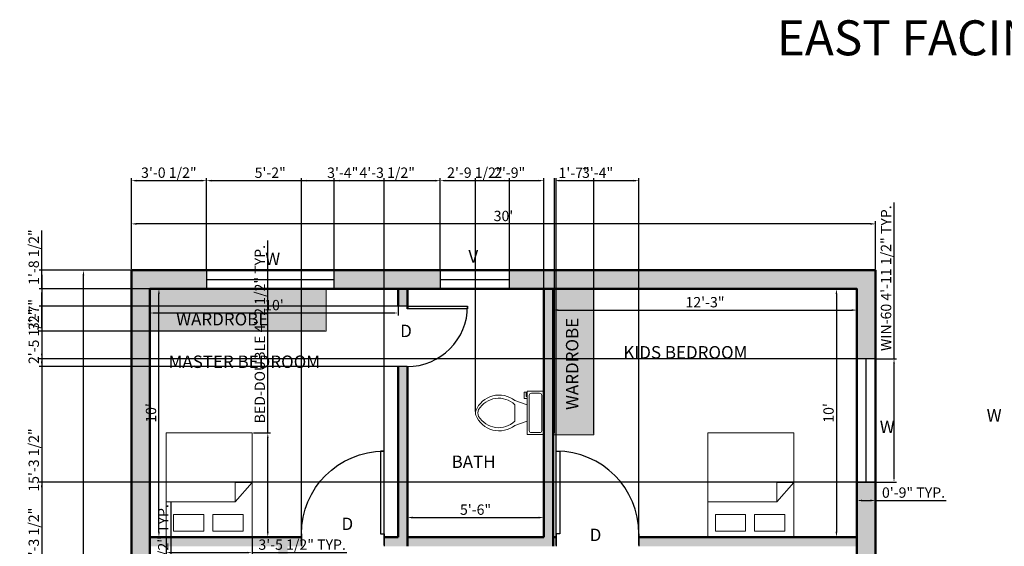
# Model space of a CAD drawing. Units: inches. Extents: x 2064 to 2999, y 1440 to 2089.
# Tile 4 of 7: x 2064 to 2540, y 1835 to 2089. Entities that reach past the tile are written whole.
import ezdxf

# ---------------------------------------------------------------- set-up
doc = ezdxf.new("R2010")
doc.units = ezdxf.units.IN
for name, color, linetype, lineweight in [('A-ANNO-DIMS', 2, 'Continuous', 18), ('A-ANNO-TEXT', 3, 'Continuous', 18), ('A-AREA-IDEN', 7, 'Continuous', 18), ('A-DOOR', 4, 'Continuous', 25), ('A-FLOR-FIXT', 9, 'Continuous', 18), ('A-FURN', 8, 'Continuous', 18), ('A-FURN-PATT', 252, 'Continuous', 13), ('A-GLAZ', 3, 'Continuous', 25), ('A-WALL', 7, 'Continuous', 50), ('A-WALL-PATT', 8, 'Continuous', 13)]:
    doc.layers.add(name, color=color, linetype=linetype, lineweight=lineweight)
doc.styles.get("Standard").update_dxf_attribs({"font": 'arial.ttf'})
doc.dimstyles.new('ISO-25', dxfattribs={"dimtxt": 5, "dimasz": 2.5, "dimexe": 1.25, "dimexo": 0.625, "dimtad": 1, "dimdec": 0, "dimlunit": 4, "dimtxsty": 'Standard', "dimcen": 2.5, "dimadec": 0, "dimazin": 0, "dimtfac": 1, "dimtdec": 0, "dimtmove": 0, "dimatfit": 3, "dimfxl": 1, "dimarcsym": 0})

# ---------------------------------------------------------------- blocks, each defined once
blk = doc.blocks.new('*U2')
for p, q in [((0, 0), (0, -6)), ((40, 0), (40, -6))]:
    blk.add_line(p, q)
blk.add_lwpolyline([(0, 0), (0, 40), (1.75, 40), (1.75, 0)], close=True)
blk.add_arc((0, 0), 40, 0, 90)
blk = doc.blocks.new('*U4')
for p, q in [((9.5, -6), (9.5, -2)), ((-10, -8.5), (-8, -8.5)), ((-10, -9.5), (-10, -8.5)), ((-7, -9.5), (-10, -9.5)), ((-8, -8.5), (-8, -8)), ((-7, -8), (-7, -9.5)), ((-4, -8), (-6, -14)), ((4, -8), (6, -14)), ((4, -14), (-4, -14))]:
    blk.add_line(p, q)
blk.add_lwpolyline([(10.5, -8), (10.5, 0), (-10.5, 0), (-10.5, -8)], close=True)
for points in [[(-9.5, -2), (-9.5, -6)], [(8.5, -1), (-8.5, -1)], [(-8.5, -7), (8.5, -7)]]:
    blk.add_lwpolyline(points)
for centre, radius, start, end in [((-8.62, -1.88), 0.884, 81.8699, 188.1301), ((8.62, -1.88), 0.884, 351.8699, 98.1301), ((-8.62, -6.12), 0.884, 171.8699, 278.1301), ((8.62, -6.12), 0.884, 261.8699, 8.1301), ((3.52, -21.58), 12.17, 141.4691, 247.9714), ((4.2, -21.82), 11.33, 136.3677, 238.9468), ((-3.52, -21.58), 12.17, 292.0284, 38.5307), ((-4.2, -21.82), 11.33, 301.053, 43.6321), ((0, -27.88), 4, 245.7318, 294.2682), ((0, -29), 4, 254.8605, 285.1395)]:
    blk.add_arc(centre, radius, start, end)
blk = doc.blocks.new('*D5')
at = {"layer": 'A-ANNO-DIMS', "color": 0, "lineweight": -2, "transparency": 16777216}
for p, q in [((2126.82, 1958.45), (2126.82, 1946.16)), ((2246.82, 1958.45), (2246.82, 1946.16)), ((2129.32, 1947.41), (2244.32, 1947.41))]:
    blk.add_line(p, q, dxfattribs=at)
at = {"layer": 'A-ANNO-DIMS', "color": 0, "transparency": 16777216}
for points in [[(2129.32, 1947.83), (2129.32, 1947), (2126.82, 1947.41)], [(2244.32, 1947.83), (2244.32, 1947), (2246.82, 1947.41)]]:
    blk.add_solid(points, dxfattribs=at)
at = {"layer": 'Defpoints', "color": 0, "transparency": 16777216}
for p in [(2126.82, 1959.07), (2246.82, 1959.07), (2246.82, 1947.41)]:
    blk.add_point(p, dxfattribs=at)
at = {"layer": 'A-ANNO-DIMS', "color": 0, "transparency": 16777216, "insert": (2186.82, 1950.59), "char_height": 5, "attachment_point": 5}
blk.add_mtext("10'", dxfattribs=at)
blk = doc.blocks.new('*D6')
at = {"layer": 'A-ANNO-DIMS', "color": 0, "lineweight": -2, "transparency": 16777216}
for p, q in [((2127.44, 1959.07), (2132.4, 1959.07)), ((2131.15, 1841.57), (2131.15, 1956.57)), ((2127.44, 1839.07), (2132.4, 1839.07))]:
    blk.add_line(p, q, dxfattribs=at)
at = {"layer": 'A-ANNO-DIMS', "color": 0, "transparency": 16777216}
for points in [[(2130.73, 1956.57), (2131.57, 1956.57), (2131.15, 1959.07)], [(2130.73, 1841.57), (2131.57, 1841.57), (2131.15, 1839.07)]]:
    blk.add_solid(points, dxfattribs=at)
at = {"layer": 'Defpoints', "color": 0, "transparency": 16777216}
for p in [(2126.82, 1959.07), (2131.15, 1959.07), (2126.82, 1839.07)]:
    blk.add_point(p, dxfattribs=at)
at = {"layer": 'A-ANNO-DIMS', "color": 0, "transparency": 16777216, "insert": (2127.97, 1899.07), "char_height": 5, "attachment_point": 5, "rotation": 90}
blk.add_mtext("10'", dxfattribs=at)
blk = doc.blocks.new('*D7')
at = {"layer": 'A-ANNO-DIMS', "color": 0, "lineweight": -2, "transparency": 16777216}
for p, q in [((2251.32, 1839.7), (2251.32, 1849.72)), ((2253.82, 1848.47), (2314.82, 1848.47)), ((2317.32, 1839.7), (2317.32, 1849.72))]:
    blk.add_line(p, q, dxfattribs=at)
at = {"layer": 'A-ANNO-DIMS', "color": 0, "transparency": 16777216}
for points in [[(2253.82, 1848.88), (2253.82, 1848.05), (2251.32, 1848.47)], [(2314.82, 1848.88), (2314.82, 1848.05), (2317.32, 1848.47)]]:
    blk.add_solid(points, dxfattribs=at)
at = {"layer": 'Defpoints', "color": 0, "transparency": 16777216}
for p in [(2317.32, 1848.47), (2251.32, 1839.07), (2317.32, 1839.07)]:
    blk.add_point(p, dxfattribs=at)
at = {"layer": 'A-ANNO-DIMS', "color": 0, "transparency": 16777216, "insert": (2284.32, 1851.65), "char_height": 5, "attachment_point": 5}
blk.add_mtext('5\'-6"', dxfattribs=at)
blk = doc.blocks.new('*D8')
at = {"layer": 'A-ANNO-DIMS', "color": 0, "lineweight": -2, "transparency": 16777216}
for p, q in [((2321.82, 1958.45), (2321.82, 1947.56)), ((2468.82, 1958.45), (2468.82, 1947.56)), ((2324.32, 1948.81), (2466.32, 1948.81))]:
    blk.add_line(p, q, dxfattribs=at)
at = {"layer": 'A-ANNO-DIMS', "color": 0, "transparency": 16777216}
for points in [[(2324.32, 1949.22), (2324.32, 1948.39), (2321.82, 1948.81)], [(2466.32, 1949.22), (2466.32, 1948.39), (2468.82, 1948.81)]]:
    blk.add_solid(points, dxfattribs=at)
at = {"layer": 'Defpoints', "color": 0, "transparency": 16777216}
for p in [(2321.82, 1959.07), (2468.82, 1959.07), (2468.82, 1948.81)]:
    blk.add_point(p, dxfattribs=at)
at = {"layer": 'A-ANNO-DIMS', "color": 0, "transparency": 16777216, "insert": (2395.32, 1951.99), "char_height": 5, "attachment_point": 5}
blk.add_mtext('12\'-3"', dxfattribs=at)
blk = doc.blocks.new('*D9')
at = {"layer": 'A-ANNO-DIMS', "color": 0, "lineweight": -2, "transparency": 16777216}
for p, q in [((2468.19, 1959.07), (2457.65, 1959.07)), ((2458.9, 1956.57), (2458.9, 1841.57)), ((2468.19, 1839.07), (2457.65, 1839.07))]:
    blk.add_line(p, q, dxfattribs=at)
at = {"layer": 'A-ANNO-DIMS', "color": 0, "transparency": 16777216}
for points in [[(2458.48, 1956.57), (2459.32, 1956.57), (2458.9, 1959.07)], [(2458.48, 1841.57), (2459.32, 1841.57), (2458.9, 1839.07)]]:
    blk.add_solid(points, dxfattribs=at)
at = {"layer": 'Defpoints', "color": 0, "transparency": 16777216}
for p in [(2468.82, 1959.07), (2458.9, 1839.07), (2468.82, 1839.07)]:
    blk.add_point(p, dxfattribs=at)
at = {"layer": 'A-ANNO-DIMS', "color": 0, "transparency": 16777216, "insert": (2455.72, 1899.07), "char_height": 5, "attachment_point": 5, "rotation": 90}
blk.add_mtext("10'", dxfattribs=at)
blk = doc.blocks.new('*D17')
at = {"layer": 'A-ANNO-DIMS', "color": 0, "lineweight": -2, "transparency": 16777216}
for p, q in [((2117.82, 1968.7), (2117.82, 1991.76)), ((2477.82, 1968.7), (2477.82, 1991.76)), ((2475.32, 1990.51), (2120.32, 1990.51))]:
    blk.add_line(p, q, dxfattribs=at)
at = {"layer": 'A-ANNO-DIMS', "color": 0, "transparency": 16777216}
for points in [[(2120.32, 1990.92), (2120.32, 1990.09), (2117.82, 1990.51)], [(2475.32, 1990.92), (2475.32, 1990.09), (2477.82, 1990.51)]]:
    blk.add_solid(points, dxfattribs=at)
at = {"layer": 'Defpoints', "color": 0, "transparency": 16777216}
for p in [(2117.82, 1990.51), (2117.82, 1968.07), (2477.82, 1968.07)]:
    blk.add_point(p, dxfattribs=at)
at = {"layer": 'A-ANNO-DIMS', "color": 0, "transparency": 16777216, "insert": (2297.82, 1993.69), "char_height": 5, "attachment_point": 5}
blk.add_mtext("30'", dxfattribs=at)
blk = doc.blocks.new('*D18')
at = {"layer": 'A-ANNO-DIMS', "color": 0, "lineweight": -2, "transparency": 16777216}
for p, q in [((2117.19, 1968.07), (2093.39, 1968.07)), ((2094.64, 1490.57), (2094.64, 1965.57)), ((2117.19, 1488.07), (2093.39, 1488.07))]:
    blk.add_line(p, q, dxfattribs=at)
at = {"layer": 'A-ANNO-DIMS', "color": 0, "transparency": 16777216}
for points in [[(2094.23, 1965.57), (2095.06, 1965.57), (2094.64, 1968.07)], [(2094.23, 1490.57), (2095.06, 1490.57), (2094.64, 1488.07)]]:
    blk.add_solid(points, dxfattribs=at)
at = {"layer": 'Defpoints', "color": 0, "transparency": 16777216}
for p in [(2094.64, 1968.07), (2117.82, 1968.07), (2117.82, 1488.07)]:
    blk.add_point(p, dxfattribs=at)
at = {"layer": 'A-ANNO-DIMS', "color": 0, "transparency": 16777216, "insert": (2091.47, 1728.07), "char_height": 5, "attachment_point": 5, "rotation": 90}
blk.add_mtext("40'", dxfattribs=at)
blk = doc.blocks.new('BED-DOUBLE')
for p, q in [((33.39, 16.96), (33.39, 26.39)), ((33.39, 26.39), (41.56, 26.39)), ((41.56, 26.39), (33.39, 16.96)), ((0, 16.96), (33.39, 16.96))]:
    blk.add_line(p, q)
for points in [[(0, 0), (41.56, 0), (41.56, 50.35), (0, 50.35)], [(3.57, 2.88), (18.22, 2.88), (18.22, 10.91), (3.57, 10.91)], [(22.49, 2.88), (37.13, 2.88), (37.13, 10.91), (22.49, 10.91)]]:
    blk.add_lwpolyline(points, close=True)
blk = doc.blocks.new('WIN-60')
blk.add_line((4.5, 0), (4.5, 59.54))
blk.add_lwpolyline([(0, 0), (9, 0), (9, 59.54), (0, 59.54)], close=True)
blk = doc.blocks.new('*D49')
at = {"layer": 'A-ANNO-DIMS', "color": 0, "lineweight": -2, "transparency": 16777216}
for p, q in [((2183.81, 1889.43), (2183.81, 1982.44)), ((2176.88, 1889.43), (2185.06, 1889.43)), ((2183.81, 1841.57), (2183.81, 1886.93)), ((2176.88, 1839.07), (2185.06, 1839.07))]:
    blk.add_line(p, q, dxfattribs=at)
at = {"layer": 'A-ANNO-DIMS', "color": 0, "transparency": 16777216}
for points in [[(2183.39, 1886.93), (2184.23, 1886.93), (2183.81, 1889.43)], [(2183.39, 1841.57), (2184.23, 1841.57), (2183.81, 1839.07)]]:
    blk.add_solid(points, dxfattribs=at)
at = {"layer": 'Defpoints', "color": 0, "transparency": 16777216}
for p in [(2176.26, 1889.43), (2183.81, 1889.43), (2176.26, 1839.07)]:
    blk.add_point(p, dxfattribs=at)
at = {"layer": 'A-ANNO-DIMS', "color": 0, "transparency": 16777216, "insert": (2180.6, 1937.18), "char_height": 5, "attachment_point": 5, "rotation": 90}
blk.add_mtext('BED-DOUBLE 4\'-2 1/2" TYP.', dxfattribs=at)
blk = doc.blocks.new('*D50')
at = {"layer": 'A-ANNO-DIMS', "color": 0, "lineweight": -2, "transparency": 16777216}
for p, q in [((2134.69, 1838.45), (2134.69, 1830.27)), ((2176.26, 1838.45), (2176.26, 1830.27)), ((2137.19, 1831.52), (2173.76, 1831.52)), ((2176.26, 1831.52), (2222.13, 1831.52))]:
    blk.add_line(p, q, dxfattribs=at)
at = {"layer": 'A-ANNO-DIMS', "color": 0, "transparency": 16777216}
for points in [[(2137.19, 1831.93), (2137.19, 1831.1), (2134.69, 1831.52)], [(2173.76, 1831.93), (2173.76, 1831.1), (2176.26, 1831.52)]]:
    blk.add_solid(points, dxfattribs=at)
at = {"layer": 'Defpoints', "color": 0, "transparency": 16777216}
for p in [(2134.69, 1839.07), (2176.26, 1839.07), (2176.26, 1831.52)]:
    blk.add_point(p, dxfattribs=at)
at = {"layer": 'A-ANNO-DIMS', "color": 0, "transparency": 16777216, "insert": (2200.44, 1834.73), "char_height": 5, "attachment_point": 5}
blk.add_mtext('3\'-5 1/2" TYP.', dxfattribs=at)
blk = doc.blocks.new('*D59')
at = {"layer": 'A-ANNO-DIMS', "color": 0, "lineweight": -2, "transparency": 16777216}
for p, q in [((2137.08, 1784.53), (2137.08, 1856.23)), ((2127.44, 1784.53), (2138.33, 1784.53)), ((2137.08, 1718.6), (2137.08, 1782.03)), ((2127.44, 1716.1), (2138.33, 1716.1))]:
    blk.add_line(p, q, dxfattribs=at)
at = {"layer": 'A-ANNO-DIMS', "color": 0, "transparency": 16777216}
for points in [[(2136.67, 1782.03), (2137.5, 1782.03), (2137.08, 1784.53)], [(2136.67, 1718.6), (2137.5, 1718.6), (2137.08, 1716.1)]]:
    blk.add_solid(points, dxfattribs=at)
at = {"layer": 'Defpoints', "color": 0, "transparency": 16777216}
for p in [(2126.82, 1784.53), (2137.08, 1784.53), (2126.82, 1716.1)]:
    blk.add_point(p, dxfattribs=at)
at = {"layer": 'A-ANNO-DIMS', "color": 0, "transparency": 16777216, "insert": (2133.87, 1821.63), "char_height": 5, "attachment_point": 5, "rotation": 90}
blk.add_mtext('WIN-68 5\'-8 1/2" TYP.', dxfattribs=at)
blk = doc.blocks.new('*D63')
at = {"layer": 'A-ANNO-DIMS', "color": 0, "lineweight": -2, "transparency": 16777216}
for p, q in [((2486.75, 1925.2), (2486.75, 2000.78)), ((2478.44, 1925.2), (2488, 1925.2)), ((2486.75, 1868.16), (2486.75, 1922.7)), ((2478.44, 1865.66), (2488, 1865.66))]:
    blk.add_line(p, q, dxfattribs=at)
at = {"layer": 'A-ANNO-DIMS', "color": 0, "transparency": 16777216}
for points in [[(2486.33, 1922.7), (2487.17, 1922.7), (2486.75, 1925.2)], [(2486.33, 1868.16), (2487.17, 1868.16), (2486.75, 1865.66)]]:
    blk.add_solid(points, dxfattribs=at)
at = {"layer": 'Defpoints', "color": 0, "transparency": 16777216}
for p in [(2477.82, 1925.2), (2486.75, 1925.2), (2477.82, 1865.66)]:
    blk.add_point(p, dxfattribs=at)
at = {"layer": 'A-ANNO-DIMS', "color": 0, "transparency": 16777216, "insert": (2483.54, 1964.24), "char_height": 5, "attachment_point": 5, "rotation": 90}
blk.add_mtext('WIN-60 4\'-11 1/2" TYP.', dxfattribs=at)
blk = doc.blocks.new('*D64')
at = {"layer": 'A-ANNO-DIMS', "color": 0, "lineweight": -2, "transparency": 16777216}
for p, q in [((2468.82, 1865.03), (2468.82, 1855.47)), ((2477.82, 1865.03), (2477.82, 1855.47)), ((2471.32, 1856.72), (2475.32, 1856.72)), ((2477.82, 1856.72), (2512.05, 1856.72))]:
    blk.add_line(p, q, dxfattribs=at)
at = {"layer": 'A-ANNO-DIMS', "color": 0, "transparency": 16777216}
for points in [[(2471.32, 1857.14), (2471.32, 1856.31), (2468.82, 1856.72)], [(2475.32, 1857.14), (2475.32, 1856.31), (2477.82, 1856.72)]]:
    blk.add_solid(points, dxfattribs=at)
at = {"layer": 'Defpoints', "color": 0, "transparency": 16777216}
for p in [(2468.82, 1865.66), (2477.82, 1865.66), (2477.82, 1856.72)]:
    blk.add_point(p, dxfattribs=at)
at = {"layer": 'A-ANNO-DIMS', "color": 0, "transparency": 16777216, "insert": (2496.18, 1859.9), "char_height": 5, "attachment_point": 5}
blk.add_mtext('0\'-9" TYP.', dxfattribs=at)
blk = doc.blocks.new('*D65')
at = {"layer": 'A-ANNO-DIMS', "color": 0, "lineweight": -2, "transparency": 16777216}
for p, q in [((2117.82, 1968.7), (2117.82, 2012.67)), ((2120.32, 2011.42), (2151.6, 2011.42)), ((2154.1, 1968.7), (2154.1, 2012.67))]:
    blk.add_line(p, q, dxfattribs=at)
at = {"layer": 'A-ANNO-DIMS', "color": 0, "transparency": 16777216}
for points in [[(2120.32, 2011.84), (2120.32, 2011), (2117.82, 2011.42)], [(2151.6, 2011.84), (2151.6, 2011), (2154.1, 2011.42)]]:
    blk.add_solid(points, dxfattribs=at)
at = {"layer": 'Defpoints', "color": 0, "transparency": 16777216}
for p in [(2154.1, 2011.42), (2117.82, 1968.07), (2154.1, 1968.07)]:
    blk.add_point(p, dxfattribs=at)
at = {"layer": 'A-ANNO-DIMS', "color": 0, "transparency": 16777216, "insert": (2135.96, 2014.63), "char_height": 5, "attachment_point": 5}
blk.add_mtext('3\'-0 1/2"', dxfattribs=at)
blk = doc.blocks.new('*D66')
at = {"layer": 'A-ANNO-DIMS', "color": 0, "lineweight": -2, "transparency": 16777216}
for p, q in [((2154.1, 1968.7), (2154.1, 2012.67)), ((2156.6, 2011.42), (2213.38, 2011.42)), ((2215.88, 1968.7), (2215.88, 2012.67))]:
    blk.add_line(p, q, dxfattribs=at)
at = {"layer": 'A-ANNO-DIMS', "color": 0, "transparency": 16777216}
for points in [[(2156.6, 2011.84), (2156.6, 2011), (2154.1, 2011.42)], [(2213.38, 2011.84), (2213.38, 2011), (2215.88, 2011.42)]]:
    blk.add_solid(points, dxfattribs=at)
at = {"layer": 'Defpoints', "color": 0, "transparency": 16777216}
for p in [(2215.88, 2011.42), (2154.1, 1968.07), (2215.88, 1968.07)]:
    blk.add_point(p, dxfattribs=at)
at = {"layer": 'A-ANNO-DIMS', "color": 0, "transparency": 16777216, "insert": (2184.99, 2014.6), "char_height": 5, "attachment_point": 5}
blk.add_mtext('5\'-2"', dxfattribs=at)
blk = doc.blocks.new('*D67')
at = {"layer": 'A-ANNO-DIMS', "color": 0, "lineweight": -2, "transparency": 16777216}
for p, q in [((2215.88, 1968.7), (2215.88, 2012.67)), ((2218.38, 2011.42), (2264.77, 2011.42)), ((2267.27, 1968.7), (2267.27, 2012.67))]:
    blk.add_line(p, q, dxfattribs=at)
at = {"layer": 'A-ANNO-DIMS', "color": 0, "transparency": 16777216}
for points in [[(2218.38, 2011.84), (2218.38, 2011), (2215.88, 2011.42)], [(2264.77, 2011.84), (2264.77, 2011), (2267.27, 2011.42)]]:
    blk.add_solid(points, dxfattribs=at)
at = {"layer": 'Defpoints', "color": 0, "transparency": 16777216}
for p in [(2267.27, 2011.42), (2215.88, 1968.07), (2267.27, 1968.07)]:
    blk.add_point(p, dxfattribs=at)
at = {"layer": 'A-ANNO-DIMS', "color": 0, "transparency": 16777216, "insert": (2241.58, 2014.63), "char_height": 5, "attachment_point": 5}
blk.add_mtext('4\'-3 1/2"', dxfattribs=at)
blk = doc.blocks.new('*D68')
at = {"layer": 'A-ANNO-DIMS', "color": 0, "lineweight": -2, "transparency": 16777216}
for p, q in [((2267.27, 1968.7), (2267.27, 2012.67)), ((2269.77, 2011.42), (2298.23, 2011.42)), ((2300.73, 1968.7), (2300.73, 2012.67))]:
    blk.add_line(p, q, dxfattribs=at)
at = {"layer": 'A-ANNO-DIMS', "color": 0, "transparency": 16777216}
for points in [[(2269.77, 2011.84), (2269.77, 2011), (2267.27, 2011.42)], [(2298.23, 2011.84), (2298.23, 2011), (2300.73, 2011.42)]]:
    blk.add_solid(points, dxfattribs=at)
at = {"layer": 'Defpoints', "color": 0, "transparency": 16777216}
for p in [(2300.73, 2011.42), (2267.27, 1968.07), (2300.73, 1968.07)]:
    blk.add_point(p, dxfattribs=at)
at = {"layer": 'A-ANNO-DIMS', "color": 0, "transparency": 16777216, "insert": (2284, 2014.63), "char_height": 5, "attachment_point": 5}
blk.add_mtext('2\'-9 1/2"', dxfattribs=at)
blk = doc.blocks.new('*D69')
at = {"layer": 'A-ANNO-DIMS', "color": 0, "lineweight": -2, "transparency": 16777216}
for p, q in [((2477.19, 1968.07), (2073.22, 1968.07)), ((2074.47, 1965.57), (2074.47, 1927.7)), ((2477.19, 1925.2), (2073.22, 1925.2))]:
    blk.add_line(p, q, dxfattribs=at)
at = {"layer": 'A-ANNO-DIMS', "color": 0, "transparency": 16777216}
for points in [[(2074.05, 1965.57), (2074.89, 1965.57), (2074.47, 1968.07)], [(2074.05, 1927.7), (2074.89, 1927.7), (2074.47, 1925.2)]]:
    blk.add_solid(points, dxfattribs=at)
at = {"layer": 'Defpoints', "color": 0, "transparency": 16777216}
for p in [(2477.82, 1968.07), (2074.47, 1925.2), (2477.82, 1925.2)]:
    blk.add_point(p, dxfattribs=at)
at = {"layer": 'A-ANNO-DIMS', "color": 0, "transparency": 16777216, "insert": (2071.29, 1946.64), "char_height": 5, "attachment_point": 5, "rotation": 90}
blk.add_mtext('3\'-7"', dxfattribs=at)
blk = doc.blocks.new('*D70')
at = {"layer": 'A-ANNO-DIMS', "color": 0, "lineweight": -2, "transparency": 16777216}
for p, q in [((2477.19, 1865.66), (2073.22, 1865.66)), ((2074.47, 1863.16), (2074.47, 1816.51)), ((2477.19, 1814.01), (2073.22, 1814.01))]:
    blk.add_line(p, q, dxfattribs=at)
at = {"layer": 'A-ANNO-DIMS', "color": 0, "transparency": 16777216}
for points in [[(2074.05, 1863.16), (2074.89, 1863.16), (2074.47, 1865.66)], [(2074.05, 1816.51), (2074.89, 1816.51), (2074.47, 1814.01)]]:
    blk.add_solid(points, dxfattribs=at)
at = {"layer": 'Defpoints', "color": 0, "transparency": 16777216}
for p in [(2477.82, 1865.66), (2074.47, 1814.01), (2477.82, 1814.01)]:
    blk.add_point(p, dxfattribs=at)
at = {"layer": 'A-ANNO-DIMS', "color": 0, "transparency": 16777216, "insert": (2071.26, 1839.83), "char_height": 5, "attachment_point": 5, "rotation": 90}
blk.add_mtext('4\'-3 1/2"', dxfattribs=at)
blk = doc.blocks.new('*D74')
at = {"layer": 'A-ANNO-DIMS', "color": 0, "lineweight": -2, "transparency": 16777216}
for p, q in [((2117.19, 1968.07), (2073.22, 1968.07)), ((2074.47, 1965.57), (2074.47, 1787.03)), ((2117.19, 1784.53), (2073.22, 1784.53))]:
    blk.add_line(p, q, dxfattribs=at)
at = {"layer": 'A-ANNO-DIMS', "color": 0, "transparency": 16777216}
for points in [[(2074.05, 1965.57), (2074.89, 1965.57), (2074.47, 1968.07)], [(2074.05, 1787.03), (2074.89, 1787.03), (2074.47, 1784.53)]]:
    blk.add_solid(points, dxfattribs=at)
at = {"layer": 'Defpoints', "color": 0, "transparency": 16777216}
for p in [(2117.82, 1968.07), (2074.47, 1784.53), (2117.82, 1784.53)]:
    blk.add_point(p, dxfattribs=at)
at = {"layer": 'A-ANNO-DIMS', "color": 0, "transparency": 16777216, "insert": (2071.26, 1876.3), "char_height": 5, "attachment_point": 5, "rotation": 90}
blk.add_mtext('15\'-3 1/2"', dxfattribs=at)
blk = doc.blocks.new('*D103')
at = {"layer": 'A-ANNO-DIMS', "color": 0, "lineweight": -2, "transparency": 16777216}
for p, q in [((2284.32, 1899.7), (2284.32, 2012.67)), ((2286.82, 2011.42), (2314.82, 2011.42)), ((2317.32, 1899.7), (2317.32, 2012.67))]:
    blk.add_line(p, q, dxfattribs=at)
at = {"layer": 'A-ANNO-DIMS', "color": 0, "transparency": 16777216}
for points in [[(2286.82, 2011.84), (2286.82, 2011), (2284.32, 2011.42)], [(2314.82, 2011.84), (2314.82, 2011), (2317.32, 2011.42)]]:
    blk.add_solid(points, dxfattribs=at)
at = {"layer": 'Defpoints', "color": 0, "transparency": 16777216}
for p in [(2317.32, 2011.42), (2284.32, 1899.07), (2317.32, 1899.07)]:
    blk.add_point(p, dxfattribs=at)
at = {"layer": 'A-ANNO-DIMS', "color": 0, "transparency": 16777216, "insert": (2300.82, 2014.6), "char_height": 5, "attachment_point": 5}
blk.add_mtext('2\'-9"', dxfattribs=at)
blk = doc.blocks.new('*D107')
at = {"layer": 'A-ANNO-DIMS', "color": 0, "lineweight": -2, "transparency": 16777216}
for p, q in [((2074.47, 1959.07), (2074.47, 1987.29)), ((2211.36, 1959.07), (2073.22, 1959.07)), ((2074.47, 1941.07), (2074.47, 1956.57)), ((2211.36, 1938.57), (2073.22, 1938.57))]:
    blk.add_line(p, q, dxfattribs=at)
at = {"layer": 'A-ANNO-DIMS', "color": 0, "transparency": 16777216}
for points in [[(2074.05, 1956.57), (2074.89, 1956.57), (2074.47, 1959.07)], [(2074.05, 1941.07), (2074.89, 1941.07), (2074.47, 1938.57)]]:
    blk.add_solid(points, dxfattribs=at)
at = {"layer": 'Defpoints', "color": 0, "transparency": 16777216}
for p in [(2074.47, 1959.07), (2211.98, 1959.07), (2211.98, 1938.57)]:
    blk.add_point(p, dxfattribs=at)
at = {"layer": 'A-ANNO-DIMS', "color": 0, "transparency": 16777216, "insert": (2071.26, 1974.43), "char_height": 5, "attachment_point": 5, "rotation": 90}
blk.add_mtext('1\'-8 1/2"', dxfattribs=at)
blk = doc.blocks.new('*D108')
at = {"layer": 'A-ANNO-DIMS', "color": 0, "lineweight": -2, "transparency": 16777216}
for p, q in [((2322.52, 1889.36), (2322.52, 2012.67)), ((2325.02, 2011.42), (2338.97, 2011.42)), ((2341.47, 1889.14), (2341.47, 2012.67))]:
    blk.add_line(p, q, dxfattribs=at)
at = {"layer": 'A-ANNO-DIMS', "color": 0, "transparency": 16777216}
for points in [[(2325.02, 2011.84), (2325.02, 2011), (2322.52, 2011.42)], [(2338.97, 2011.84), (2338.97, 2011), (2341.47, 2011.42)]]:
    blk.add_solid(points, dxfattribs=at)
at = {"layer": 'Defpoints', "color": 0, "transparency": 16777216}
for p in [(2341.47, 2011.42), (2322.52, 1888.74), (2341.47, 1888.51)]:
    blk.add_point(p, dxfattribs=at)
at = {"layer": 'A-ANNO-DIMS', "color": 0, "transparency": 16777216, "insert": (2331.99, 2014.56), "char_height": 5, "attachment_point": 5}
blk.add_mtext('1\'-7"', dxfattribs=at)
blk = doc.blocks.new('*D110')
at = {"layer": 'A-ANNO-DIMS', "color": 0, "lineweight": -2, "transparency": 16777216}
for p, q in [((2200.07, 1835.2), (2200.07, 2012.67)), ((2202.57, 2011.42), (2237.57, 2011.42)), ((2240.07, 1835.2), (2240.07, 2012.67))]:
    blk.add_line(p, q, dxfattribs=at)
at = {"layer": 'A-ANNO-DIMS', "color": 0, "transparency": 16777216}
for points in [[(2202.57, 2011.84), (2202.57, 2011), (2200.07, 2011.42)], [(2237.57, 2011.84), (2237.57, 2011), (2240.07, 2011.42)]]:
    blk.add_solid(points, dxfattribs=at)
at = {"layer": 'Defpoints', "color": 0, "transparency": 16777216}
for p in [(2240.07, 2011.42), (2200.07, 1834.57), (2240.07, 1834.57)]:
    blk.add_point(p, dxfattribs=at)
at = {"layer": 'A-ANNO-DIMS', "color": 0, "transparency": 16777216, "insert": (2220.07, 2014.6), "char_height": 5, "attachment_point": 5}
blk.add_mtext('3\'-4"', dxfattribs=at)
blk = doc.blocks.new('*D111')
at = {"layer": 'A-ANNO-DIMS', "color": 0, "lineweight": -2, "transparency": 16777216}
for p, q in [((2323.36, 1835.2), (2323.36, 2012.67)), ((2325.86, 2011.42), (2360.86, 2011.42)), ((2363.36, 1835.2), (2363.36, 2012.67))]:
    blk.add_line(p, q, dxfattribs=at)
at = {"layer": 'A-ANNO-DIMS', "color": 0, "transparency": 16777216}
for points in [[(2325.86, 2011.84), (2325.86, 2011), (2323.36, 2011.42)], [(2360.86, 2011.84), (2360.86, 2011), (2363.36, 2011.42)]]:
    blk.add_solid(points, dxfattribs=at)
at = {"layer": 'Defpoints', "color": 0, "transparency": 16777216}
for p in [(2363.36, 2011.42), (2323.36, 1834.57), (2363.36, 1834.57)]:
    blk.add_point(p, dxfattribs=at)
at = {"layer": 'A-ANNO-DIMS', "color": 0, "transparency": 16777216, "insert": (2343.36, 2014.6), "char_height": 5, "attachment_point": 5}
blk.add_mtext('3\'-4"', dxfattribs=at)
blk = doc.blocks.new('*D112')
at = {"layer": 'A-ANNO-DIMS', "color": 0, "lineweight": -2, "transparency": 16777216}
for p, q in [((2250.59, 1950.75), (2073.22, 1950.75)), ((2074.47, 1948.25), (2074.47, 1923.96)), ((2250.69, 1921.46), (2073.22, 1921.46))]:
    blk.add_line(p, q, dxfattribs=at)
at = {"layer": 'A-ANNO-DIMS', "color": 0, "transparency": 16777216}
for points in [[(2074.05, 1948.25), (2074.89, 1948.25), (2074.47, 1950.75)], [(2074.05, 1923.96), (2074.89, 1923.96), (2074.47, 1921.46)]]:
    blk.add_solid(points, dxfattribs=at)
at = {"layer": 'Defpoints', "color": 0, "transparency": 16777216}
for p in [(2251.21, 1950.75), (2074.47, 1921.46), (2251.32, 1921.46)]:
    blk.add_point(p, dxfattribs=at)
at = {"layer": 'A-ANNO-DIMS', "color": 0, "transparency": 16777216, "insert": (2071.26, 1936.11), "char_height": 5, "attachment_point": 5, "rotation": 90}
blk.add_mtext('2\'-5 1/2"', dxfattribs=at)

msp = doc.modelspace()

# ---------------------------------------------------------------- hatches: boundary and pattern name
at = {"layer": 'A-FURN-PATT'}
h = msp.add_hatch(color=256, dxfattribs=at)
h.dxf.hatch_style = 1
h.paths.add_polyline_path([(2211.98, 1959.07), (2126.82, 1959.07), (2126.82, 1938.57), (2211.98, 1938.57)])
h.paths.add_polyline_path([(2669.87, 1959.07), (2646.96, 1959.07), (2646.96, 1892.49), (2669.87, 1892.49)])
h.paths.add_polyline_path([(2468.82, 1668.53), (2348.82, 1668.53), (2348.82, 1638.07), (2468.82, 1638.07)])
h.paths.add_polyline_path([(2891.87, 1667.99), (2780.13, 1667.99), (2780.13, 1638.07), (2891.87, 1638.07)])
h.paths.add_polyline_path([(2854.27, 1658.75), (2854.27, 1650.97), (2859.31, 1650.97), (2859.31, 1658.75), (2862.16, 1658.75), (2862.16, 1650.97), (2867.47, 1650.97), (2867.47, 1658.75), (2870.33, 1658.75), (2870.33, 1650.97), (2879.45, 1650.97), (2879.45, 1658.75), (2882.31, 1658.75), (2882.31, 1643.24), (2879.45, 1643.24), (2879.45, 1650.97), (2870.33, 1650.97), (2870.33, 1643.24), (2867.47, 1643.24), (2867.47, 1650.97), (2862.16, 1650.97), (2862.16, 1643.24), (2859.31, 1643.24), (2859.31, 1650.97), (2854.27, 1650.97), (2854.27, 1643.24), (2851.41, 1643.24), (2851.41, 1650.97), (2845.97, 1650.97), (2845.97, 1643.24), (2843.11, 1643.24), (2843.11, 1650.97), (2839.98, 1650.97), (2839.98, 1643.24), (2837.12, 1643.24), (2837.12, 1650.97), (2831.27, 1650.97), (2831.27, 1643.24), (2828.41, 1643.24), (2828.41, 1650.97), (2823.78, 1650.97), (2823.78, 1643.24), (2820.92, 1643.24), (2820.92, 1650.97), (2816.56, 1650.97), (2816.56, 1641.66), (2813.71, 1641.66), (2813.71, 1650.97), (2808.81, 1650.97), (2808.81, 1641.66), (2805.95, 1641.66), (2805.95, 1650.97), (2801.73, 1650.97), (2801.73, 1641.66), (2798.87, 1641.66), (2798.87, 1650.97), (2794.92, 1650.97), (2794.92, 1643.24), (2792.06, 1643.24), (2792.06, 1658.75), (2794.92, 1658.75), (2794.92, 1650.97), (2798.87, 1650.97), (2798.87, 1657.16), (2801.73, 1657.16), (2801.73, 1650.97), (2805.95, 1650.97), (2805.95, 1657.16), (2808.81, 1657.16), (2808.81, 1650.97), (2813.71, 1650.97), (2813.71, 1657.16), (2816.56, 1657.16), (2816.56, 1650.97), (2820.92, 1650.97), (2820.92, 1658.75), (2823.78, 1658.75), (2823.78, 1650.97), (2828.41, 1650.97), (2828.41, 1658.75), (2831.27, 1658.75), (2831.27, 1650.97), (2837.12, 1650.97), (2837.12, 1658.75), (2839.98, 1658.75), (2839.98, 1650.97), (2843.11, 1650.97), (2843.11, 1658.75), (2845.97, 1658.75), (2845.97, 1650.97), (2851.41, 1650.97), (2851.41, 1658.75)], flags=16)
h.paths.add_polyline_path([(2665.84, 1899.31), (2665.84, 1951.8), (2653.45, 1951.8), (2653.45, 1899.31)], flags=24)
h.paths.add_polyline_path([(2565.91, 1921.55), (2649.69, 1921.55), (2649.69, 1933.95), (2565.91, 1933.95)], flags=9)
h.paths.add_polyline_path([(2402.8, 1649), (2414.4, 1649), (2414.4, 1659.3), (2402.8, 1659.3)], flags=24)
h = msp.add_hatch(color=256, dxfattribs=at)
h.dxf.hatch_style = 1
h.paths.add_polyline_path([(2341.47, 1959.07), (2321.82, 1959.07), (2321.82, 1888.51), (2341.47, 1888.51)])
h.paths.add_polyline_path([(2337.44, 1898.9), (2337.44, 1951.39), (2325.04, 1951.39), (2325.04, 1898.9)], flags=24)
at = {"layer": 'A-WALL-PATT'}
h = msp.add_hatch(color=256, dxfattribs=at)
h.dxf.hatch_style = 1
h.paths.add_polyline_path([(2267.27, 1968.07), (2215.88, 1968.07), (2215.88, 1959.07), (2246.82, 1959.07), (2267.27, 1959.07)])
h.paths.add_polyline_path([(2477.82, 1968.07), (2300.73, 1968.07), (2300.73, 1959.07), (2317.32, 1959.07), (2468.82, 1959.07), (2468.82, 1925.2), (2477.82, 1925.2)])
h.paths.add_polyline_path([(2154.1, 1968.07), (2117.82, 1968.07), (2117.82, 1784.53), (2126.82, 1784.53), (2126.82, 1959.07), (2154.1, 1959.07)])
h.paths.add_polyline_path([(2126.82, 1716.1), (2117.82, 1716.1), (2117.82, 1685.76), (2126.82, 1685.76)])
h.paths.add_polyline_path([(2126.82, 1617.33), (2117.82, 1617.33), (2117.82, 1589.89), (2126.82, 1589.89)])
h.paths.add_polyline_path([(2273.05, 1497.07), (2228.82, 1497.07), (2126.82, 1497.07), (2126.82, 1521.07), (2126.82, 1521.46), (2117.82, 1521.46), (2117.82, 1488.07), (2273.05, 1488.07)])
h.paths.add_polyline_path([(2409.19, 1494.07, -0.01877), (2409.3, 1497.07), (2356.92, 1497.07), (2356.92, 1488.07), (2409.19, 1488.07)])
h.paths.add_polyline_path([(2468.82, 1638.07), (2348.82, 1638.07), (2348.82, 1668.53), (2348.82, 1710.05), (2344.32, 1710.05), (2344.32, 1633.57), (2468.82, 1633.57)])
h.paths.add_polyline_path([(2228.82, 1567.84), (2224.32, 1567.84), (2224.32, 1497.07), (2228.82, 1497.07)])
h.paths.add_polyline_path([(2477.82, 1781.8), (2468.82, 1781.8), (2468.82, 1762.57), (2468.82, 1728.07), (2477.82, 1728.07)])
h.paths.add_polyline_path([(2468.82, 1762.57), (2372.82, 1762.57), (2372.82, 1801.78), (2368.32, 1801.78), (2368.32, 1758.07), (2468.82, 1758.07)])
h.paths.add_polyline_path([(2477.82, 1865.66), (2468.82, 1865.66), (2468.82, 1814.01), (2477.82, 1814.01)])
h.paths.add_polyline_path([(2321.82, 1959.07), (2317.32, 1959.07), (2317.32, 1839.07), (2251.32, 1839.07), (2251.32, 1834.57), (2321.82, 1834.57)])
h.paths.add_polyline_path([(2200.07, 1839.07), (2126.82, 1839.07), (2126.82, 1834.57), (2200.07, 1834.57)])
h.paths.add_polyline_path([(2193.43, 1834.57), (2188.93, 1834.57), (2188.93, 1710.22), (2193.43, 1710.22)])
h.paths.add_polyline_path([(2251.32, 1959.07), (2246.82, 1959.07), (2246.82, 1950.75), (2251.21, 1950.75), (2251.32, 1950.75)])
h.paths.add_polyline_path([(2251.32, 1921.46), (2246.82, 1921.46), (2246.82, 1839.07), (2240.07, 1839.07), (2240.07, 1834.57), (2251.32, 1834.57), (2251.32, 1839.07)])
h.paths.add_polyline_path([(2468.82, 1839.07), (2363.36, 1839.07), (2363.36, 1834.57), (2468.82, 1834.57)])
h.paths.add_polyline_path([(2323.36, 1839.07), (2321.82, 1839.07), (2321.82, 1834.57), (2323.36, 1834.57)])
h = msp.add_hatch(color=256, dxfattribs=at)
h.dxf.hatch_style = 1
h.paths.add_polyline_path([(2449.19, 1497.07), (2449.19, 1494.07), (2449.19, 1488.07), (2468.82, 1488.07), (2468.82, 1497.07)])
h.paths.add_polyline_path([(2468.82, 1488.07), (2477.82, 1488.07), (2477.82, 1668.53), (2468.82, 1668.53)])
h.paths.add_polyline_path([(2454.62, 1692.05), (2454.62, 1703.66), (2444.32, 1703.66), (2444.32, 1692.05)], flags=9)
h.paths.add_polyline_path([(2167.39, 1527.81), (2183.8, 1527.81), (2183.8, 1538.12), (2167.39, 1538.12)], flags=9)
h.paths.add_polyline_path([(2343.08, 1527.75), (2354.68, 1527.75), (2354.68, 1538.06), (2343.08, 1538.06)], flags=9)
h.paths.add_polyline_path([(2462.54, 1554.96), (2462.54, 1575.25), (2452.24, 1575.25), (2452.24, 1554.96)], flags=9)
h.paths.add_polyline_path([(2140.63, 1624.84), (2140.63, 1645.13), (2130.32, 1645.13), (2130.32, 1624.84)], flags=9)
h.paths.add_polyline_path([(2137.9, 1938.01), (2190.4, 1938.01), (2190.4, 1950.4), (2137.9, 1950.4)], flags=9)
h.paths.add_polyline_path([(2337.44, 1898.9), (2337.44, 1951.39), (2325.04, 1951.39), (2325.04, 1898.9)], flags=9)
h.paths.add_polyline_path([(2380.15, 1768.58), (2405.57, 1768.58), (2405.57, 1780.97), (2380.15, 1780.97)], flags=9)
h.paths.add_polyline_path([(2370.32, 1679.42), (2432.16, 1679.42), (2432.16, 1691.82), (2370.32, 1691.82)], flags=9)
h.paths.add_polyline_path([(2322.2, 1541.98), (2382.63, 1541.98), (2382.63, 1554.37), (2322.2, 1554.37)], flags=9)
h.paths.add_polyline_path([(2153.83, 1534.75), (2193.72, 1534.75), (2193.72, 1547.14), (2153.83, 1547.14)], flags=9)
h.paths.add_polyline_path([(2162.47, 1614.19), (2217.78, 1614.19), (2217.78, 1626.58), (2162.47, 1626.58)], flags=9)
h.paths.add_polyline_path([(2217.9, 1723.52), (2261.07, 1723.52), (2261.07, 1735.92), (2217.9, 1735.92)], flags=9)
h.paths.add_polyline_path([(2270.61, 1869.16), (2296.03, 1869.16), (2296.03, 1881.55), (2270.61, 1881.55)], flags=9)
h.paths.add_polyline_path([(2353.7, 1922), (2422.07, 1922), (2422.07, 1934.4), (2353.7, 1934.4)], flags=9)
h.paths.add_polyline_path([(2133.7, 1917.44), (2217.48, 1917.44), (2217.48, 1929.83), (2133.7, 1929.83)], flags=9)

# ---------------------------------------------------------------- linework, layer by layer
at = {"layer": 'A-FURN'}
for points in [[(2126.82, 1959.07), (2211.98, 1959.07), (2211.98, 1938.57), (2126.82, 1938.57)], [(2321.82, 1888.51), (2341.47, 1888.51), (2341.47, 1959.07), (2321.82, 1959.07)]]:
    msp.add_lwpolyline(points, close=True, dxfattribs=at)
at = {"layer": 'A-GLAZ'}
for p, q in [((2154.1, 1963.57), (2215.88, 1963.57)), ((2267.27, 1963.57), (2300.73, 1963.57))]:
    msp.add_line(p, q, dxfattribs=at)
for points in [[(2154.1, 1959.07), (2215.88, 1959.07), (2215.88, 1968.07), (2154.1, 1968.07)], [(2267.27, 1959.07), (2300.73, 1959.07), (2300.73, 1968.07), (2267.27, 1968.07)]]:
    msp.add_lwpolyline(points, close=True, dxfattribs=at)
at = {"layer": 'A-WALL'}
for p, q in [((2117.82, 1968.07), (2477.82, 1968.07)), ((2117.82, 1488.07), (2117.82, 1968.07)), ((2477.82, 1968.07), (2477.82, 1488.07)), ((2126.82, 1959.07), (2246.82, 1959.07)), ((2246.82, 1959.07), (2246.82, 1950.75)), ((2251.32, 1959.07), (2251.32, 1949.47)), ((2251.32, 1959.07), (2317.32, 1959.07)), ((2317.32, 1959.07), (2317.32, 1839.07)), ((2321.82, 1959.07), (2321.82, 1834.57)), ((2246.82, 1921.46), (2246.82, 1839.07)), ((2251.32, 1921.46), (2251.32, 1834.57)), ((2200.07, 1839.07), (2126.82, 1839.07)), ((2246.82, 1839.07), (2240.07, 1839.07)), ((2317.32, 1839.07), (2251.32, 1839.07)), ((2321.82, 1839.07), (2323.36, 1839.07)), ((2363.36, 1839.07), (2468.82, 1839.07))]:
    msp.add_line(p, q, dxfattribs=at)
for points in [[(2449.19, 1488.07), (2477.82, 1488.07), (2477.82, 1968.07), (2117.82, 1968.07), (2117.82, 1488.07), (2409.19, 1488.07)], [(2447.44, 1497.07), (2468.82, 1497.07), (2468.82, 1959.07), (2126.82, 1959.07), (2126.82, 1497.07), (2409.3, 1497.07)]]:
    msp.add_lwpolyline(points, dxfattribs=at)

# ---------------------------------------------------------------- block references
at = {"layer": 'A-DOOR', "xscale": 0.7321075539063999, "yscale": 0.7321075539063999, "zscale": 0.7321075539063999, "rotation": 270}
msp.add_blockref('*U2', (2251.21, 1950.75), dxfattribs=at)
at = {"layer": 'A-DOOR', "xscale": -1}
msp.add_blockref('*U2', (2240.07, 1840.57), dxfattribs=at)
at = {"layer": 'A-DOOR'}
msp.add_blockref('*U2', (2323.36, 1840.57), dxfattribs=at)
at = {"layer": 'A-FLOR-FIXT', "rotation": 270}
msp.add_blockref('*U4', (2317.32, 1899.07), dxfattribs=at)
at = {"layer": 'A-FURN'}
for p in [(2134.7, 1839.07), (2396.75, 1839.07)]:
    msp.add_blockref('BED-DOUBLE', p, dxfattribs=at)
at = {"layer": 'A-GLAZ'}
msp.add_blockref('WIN-60', (2468.82, 1865.65), dxfattribs=at)

# ---------------------------------------------------------------- texts
at = {"layer": 'A-ANNO-TEXT', "attachment_point": 1}
for s, width, gutter_width, heights, insert, char_height in [('EAST FACING HOUSE', 429.6774, 84.65, [17.52], (2430, 2088.96), 16.9292), ('V', 152.6727, 30.08, [0], (2280.86, 1977.84), 6.02), ('W', 152.6727, 30.08, [0], (2182.59, 1976.61), 6.02), ('D', 152.6727, 30.08, [0], (2247.86, 1941.75), 6.02), ('W', 152.6727, 30.08, [0], (2531.58, 1900.91), 6.02), ('W', 152.6727, 30.08, [0], (2479.86, 1895.39), 6.02), ('D', 152.6727, 30.08, [0], (2219.48, 1848.45), 6.02), ('D', 152.6727, 30.08, [0], (2339.53, 1843.1), 6.02)]:
    msp.add_mtext_dynamic_manual_height_columns(s, width=width, gutter_width=gutter_width, heights=heights, dxfattribs=dict(at, insert=insert, char_height=char_height))
at = {"layer": 'A-AREA-IDEN', "attachment_point": 1}
for s, insert, char_height in [('WARDROBE', (2139.51, 1947.41), 6.015), ('KIDS BEDROOM', (2355.81, 1931.41), 6.0153), ('MASTER BEDROOM', (2135.83, 1926.84), 6.0153), ('BATH', (2272.73, 1878.46), 6.015)]:
    msp.add_mtext_dynamic_manual_height_columns(s, width=152.6727, gutter_width=30.08, heights=[0], dxfattribs=dict(at, insert=insert, char_height=char_height))
at = {"layer": 'A-AREA-IDEN', "insert": (2328.03, 1900.5), "char_height": 6.015, "attachment_point": 1, "rotation": 90}
msp.add_mtext_dynamic_manual_height_columns('WARDROBE', width=152.6727, gutter_width=30.08, heights=[0], dxfattribs=at)

# ---------------------------------------------------------------- dimensions: what is measured, and where the dimension line sits
at = {"layer": 'A-ANNO-DIMS'}
for base, p1, p2, override, picture, middle in [((2154.1, 2011.42), (2117.82, 1968.07), (2154.1, 1968.07), {"dimdec": 1, "dimlfac": 1, "dimrnd": 0, "dimzin": 1, "dimdsep": 46, "dimlunit": 4, "dimfrac": 2}, '*D65', (2135.96, 2014.63)), ((2267.27, 2011.42), (2215.88, 1968.07), (2267.27, 1968.07), {"dimdec": 1, "dimlfac": 1, "dimrnd": 0, "dimzin": 1, "dimdsep": 46, "dimlunit": 4, "dimfrac": 2}, '*D67', (2241.58, 2014.63)), ((2300.73, 2011.42), (2267.27, 1968.07), (2300.73, 1968.07), {"dimdec": 1, "dimlfac": 1, "dimrnd": 0, "dimzin": 1, "dimdsep": 46, "dimlunit": 4, "dimfrac": 2}, '*D68', (2284, 2014.63)), ((2215.88, 2011.42), (2154.1, 1968.07), (2215.88, 1968.07), {"dimdec": 1, "dimlfac": 1, "dimrnd": 0, "dimzin": 1, "dimdsep": 46, "dimlunit": 4, "dimfrac": 2}, '*D66', (2184.99, 2014.6)), ((2240.07, 2011.42), (2200.07, 1834.57), (2240.07, 1834.57), {"dimdec": 1, "dimlfac": 1, "dimrnd": 0, "dimzin": 1, "dimdsep": 46, "dimlunit": 4, "dimfrac": 2}, '*D110', (2220.07, 2014.6)), ((2317.32, 2011.42), (2284.32, 1899.07), (2317.32, 1899.07), {"dimdec": 1, "dimlfac": 1, "dimrnd": 0, "dimzin": 1, "dimdsep": 46, "dimlunit": 4, "dimfrac": 2}, '*D103', (2300.82, 2014.6)), ((2341.4683, 2011.4209), (2322.5163, 1888.7364), (2341.4683, 1888.5114), {"dimdec": 1, "dimlfac": 1, "dimrnd": 0, "dimzin": 1, "dimdsep": 46, "dimlunit": 4, "dimfrac": 2}, '*D108', (2331.9923, 2014.5562)), ((2363.36, 2011.42), (2323.36, 1834.57), (2363.36, 1834.57), {"dimdec": 1, "dimlfac": 1, "dimrnd": 0, "dimzin": 1, "dimdsep": 46, "dimlunit": 4, "dimfrac": 2}, '*D111', (2343.36, 2014.6)), ((2117.82, 1990.51), (2477.82, 1968.07), (2117.82, 1968.07), {"dimclrd": 0, "dimclre": 0, "dimclrt": 0}, '*D17', (2297.82, 1993.69)), ((2246.82, 1947.41), (2126.82, 1959.07), (2246.82, 1959.07), {"dimclrd": 0, "dimclre": 0, "dimclrt": 0}, '*D5', (2186.82, 1950.59)), ((2468.82, 1948.81), (2321.82, 1959.07), (2468.82, 1959.07), {"dimclrd": 0, "dimclre": 0, "dimclrt": 0}, '*D8', (2395.32, 1951.99)), ((2317.32, 1848.47), (2251.32, 1839.07), (2317.32, 1839.07), {"dimclrd": 0, "dimclre": 0, "dimclrt": 0}, '*D7', (2284.32, 1851.65))]:
    dim = msp.add_linear_dim(base=base, p1=p1, p2=p2, dimstyle='ISO-25', override=override, dxfattribs=at)
    dim.commit()
    dim.dimension.update_dxf_attribs({"geometry": picture, "text_midpoint": middle})
for base, p1, p2, text, picture, middle in [((2486.75, 1925.2), (2477.82, 1865.66), (2477.82, 1925.2), 'WIN-60 <> TYP.', '*D63', (2483.54, 1964.24)), ((2183.81, 1889.43), (2176.26, 1839.07), (2176.26, 1889.43), 'BED-DOUBLE <> TYP.', '*D49', (2180.6, 1937.18)), ((2137.08, 1784.53), (2126.82, 1716.1), (2126.82, 1784.53), 'WIN-68 <> TYP.', '*D59', (2133.87, 1821.63))]:
    dim = msp.add_linear_dim(base=base, p1=p1, p2=p2, angle=90, text=text, dimstyle='ISO-25', override={"dimdec": 1, "dimrnd": 0, "dimzin": 1, "dimlunit": 4, "dimfrac": 2}, dxfattribs=at)
    dim.commit()
    dim.dimension.update_dxf_attribs({"geometry": picture, "text_midpoint": middle})
for base, p1, p2, override, picture, middle in [((2074.47, 1959.07), (2211.98, 1938.57), (2211.98, 1959.07), {"dimdec": 1, "dimlfac": 1, "dimrnd": 0, "dimzin": 1, "dimdsep": 46, "dimlunit": 4, "dimfrac": 2}, '*D107', (2071.26, 1974.43)), ((2074.47, 1784.53), (2117.82, 1968.07), (2117.82, 1784.53), {"dimdec": 1, "dimlfac": 1, "dimrnd": 0, "dimzin": 1, "dimdsep": 46, "dimlunit": 4, "dimfrac": 2}, '*D74', (2071.26, 1876.3)), ((2074.47, 1925.2), (2477.82, 1968.07), (2477.82, 1925.2), {"dimdec": 1, "dimlfac": 1, "dimrnd": 0, "dimzin": 1, "dimdsep": 46, "dimlunit": 4, "dimfrac": 2}, '*D69', (2071.29, 1946.64)), ((2094.64, 1968.07), (2117.82, 1488.07), (2117.82, 1968.07), {"dimclrd": 0, "dimclre": 0, "dimclrt": 0}, '*D18', (2091.47, 1728.07)), ((2131.15, 1959.07), (2126.82, 1839.07), (2126.82, 1959.07), {"dimclrd": 0, "dimclre": 0, "dimclrt": 0}, '*D6', (2127.97, 1899.07)), ((2458.9, 1839.07), (2468.82, 1959.07), (2468.82, 1839.07), {"dimclrd": 0, "dimclre": 0, "dimclrt": 0}, '*D9', (2455.72, 1899.07)), ((2074.47, 1921.46), (2251.21, 1950.75), (2251.32, 1921.46), {"dimdec": 1, "dimlfac": 1, "dimrnd": 0, "dimzin": 1, "dimdsep": 46, "dimlunit": 4, "dimfrac": 2}, '*D112', (2071.26, 1936.11)), ((2074.4687, 1814.0143), (2477.8187, 1865.6554), (2477.8187, 1814.0143), {"dimdec": 1, "dimlfac": 1, "dimrnd": 0, "dimzin": 1, "dimdsep": 46, "dimlunit": 4, "dimfrac": 2}, '*D70', (2071.2567, 1839.8348))]:
    dim = msp.add_linear_dim(base=base, p1=p1, p2=p2, angle=90, dimstyle='ISO-25', override=override, dxfattribs=at)
    dim.commit()
    dim.dimension.update_dxf_attribs({"geometry": picture, "text_midpoint": middle})
for base, p1, p2, picture, middle in [((2477.82, 1856.72), (2468.82, 1865.66), (2477.82, 1865.66), '*D64', (2496.18, 1859.9)), ((2176.26, 1831.52), (2134.69, 1839.07), (2176.26, 1839.07), '*D50', (2200.44, 1834.73))]:
    dim = msp.add_linear_dim(base=base, p1=p1, p2=p2, text='<> TYP.', dimstyle='ISO-25', override={"dimdec": 1, "dimrnd": 0, "dimzin": 1, "dimlunit": 4, "dimfrac": 2}, dxfattribs=at)
    dim.commit()
    dim.dimension.update_dxf_attribs({"geometry": picture, "text_midpoint": middle})

doc.saveas('drawing.dxf')
